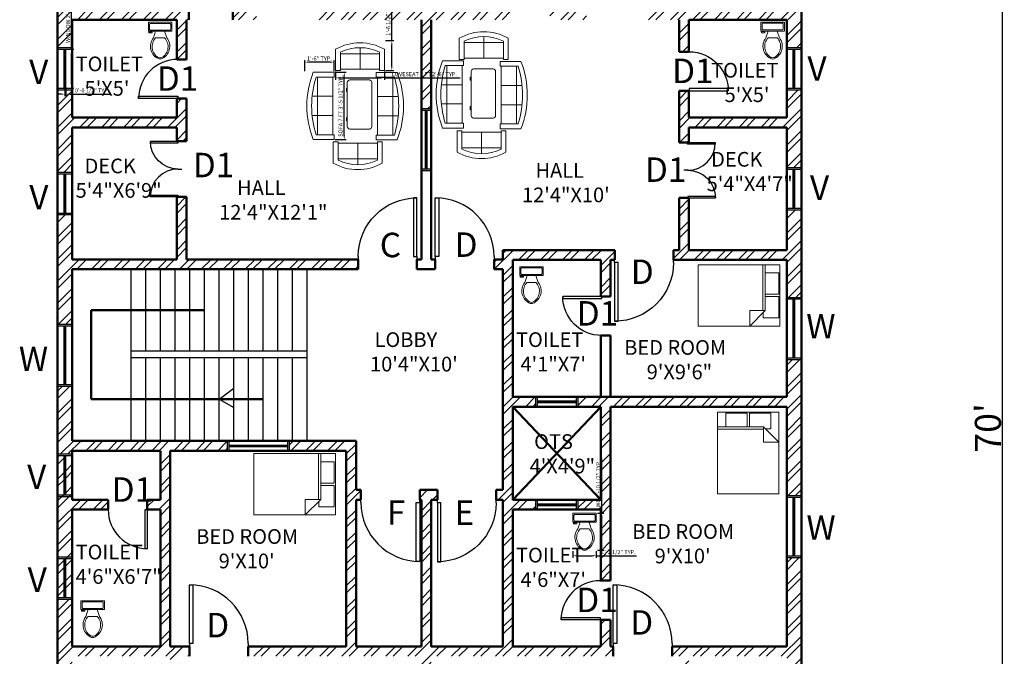
# Model space of a CAD drawing. Units: inches. Extents: x -31438 to -28352, y 12489 to 13610.
# Tile 2 of 5: x -31438 to -30834, y 12848 to 13238. Entities that reach past the tile are written whole.
import ezdxf

# ---------------------------------------------------------------- set-up
doc = ezdxf.new("R2010")
doc.units = ezdxf.units.IN
for name, color, linetype, lineweight in [('A-ANNO-DIMS', 2, 'Continuous', 18), ('A-ANNO-TEXT', 7, 'Continuous', 18), ('A-AREA-IDEN', 3, 'Continuous', 18), ('A-DOOR', 3, 'Continuous', 25), ('A-FLOR-FIXT', 9, 'Continuous', 18), ('A-FLOR-STRS', 6, 'Continuous', 25), ('A-FURN', 8, 'Continuous', 18), ('A-GLAZ', 4, 'Continuous', 25), ('A-WALL', 7, 'Continuous', 50), ('A-WALL-PATT', 8, 'Continuous', 13)]:
    doc.layers.add(name, color=color, linetype=linetype, lineweight=lineweight)
doc.styles.get("Standard").update_dxf_attribs({"font": 'arial.ttf'})
doc.dimstyles.new('ISO-25', dxfattribs={"dimtxt": 2.5, "dimasz": 2.5, "dimexe": 1.25, "dimexo": 0.625, "dimtad": 1, "dimdec": 0, "dimlunit": 3, "dimtxsty": 'Standard', "dimcen": 2.5, "dimadec": 0, "dimazin": 0, "dimtfac": 1, "dimtdec": 0, "dimtmove": 0, "dimatfit": 3, "dimfxl": 1, "dimarcsym": 0})

# ---------------------------------------------------------------- blocks, each defined once
blk = doc.blocks.new('*U8')
for p, q in [((0, 0), (0, -100)), ((750, 0), (750, -100))]:
    blk.add_line(p, q)
blk.add_lwpolyline([(0, 0), (0, 750), (43.75, 750), (43.75, 0)], close=True)
blk.add_arc((0, 0), 750, 0, 90)
blk = doc.blocks.new('Bed - Queen')
for p, q in [((0, -80.00003), (0, 0)), ((0, 0), (59.99999, 0)), ((59.99999, 0), (59.99999, -80.00003)), ((7.99999, -1.2), (28.79998, -1.2)), ((7.99999, -14.4), (7.99999, -1.2)), ((28.79998, -1.2), (28.79998, -14.4)), ((31.19999, -1.2), (51.99999, -1.2)), ((31.19999, -14.4), (31.19999, -1.2)), ((51.99999, -1.2), (51.99999, -16.4)), ((0, -14.4), (44.8, -14.4)), ((44.8, -16.8), (0, -16.8)), ((59.99999, -29.6), (44.8, -14.4)), ((44.8, -14.4), (44.8, -29.6)), ((51.99999, -16.4), (46.79936, -16.4)), ((44.8, -29.6), (59.99999, -29.6)), ((59.99999, -80.00003), (0, -80.00003))]:
    blk.add_line(p, q)
blk = doc.blocks.new('Desk - 30 x 60 in.')
for p, q in [((-26.999995, 0), (26.999995, 0)), ((-29.999995, -27), (-29.999995, -3)), ((29.999995, -3), (29.999995, -27)), ((26.999995, -30), (-26.999995, -30)), ((-20.000005, -30), (-20.000005, -31)), ((-20.000005, -31), (-16.000005, -31)), ((-16.000005, -31), (-16.000005, -30)), ((15.999995, -31), (15.999995, -30)), ((19.999995, -31), (15.999995, -31)), ((19.999995, -30), (19.999995, -31))]:
    blk.add_line(p, q)
for centre, start, end in [((-26.499995, -3.5), 98.1301, 171.8699), ((26.499995, -3.5), 8.130102, 81.8699), ((-26.499995, -26.5), 188.1301, 261.8699), ((26.499995, -26.5), 278.1301, 351.8699)]:
    blk.add_arc(centre, 3.535534, start, end)
blk = doc.blocks.new('Sofa - Roundback 7 ft.')
for p, q in [((-36.000027, -34), (-36.000027, -11.4696)), ((-12.00002, -32.4421), (-12.00003, -6.5971)), ((11.99997, -32.4421), (11.99998, -6.5971)), ((35.99998, -34), (35.99998, -11.4696)), ((-35.999844, -13.3819), (35.9998, -13.3819)), ((-36.000027, -32.4421), (35.99998, -32.4421))]:
    blk.add_line(p, q)
for points in [[(-36.000027, -34), (-42.000027, -34), (-42.000027, -8)], [(41.99998, -8), (41.99998, -34), (35.99998, -34)]]:
    blk.add_lwpolyline(points)
for centre, radius, start, end in [((0, -114.25), 114.25, 68.43141, 111.5686), ((-0.00001, -127.1968), 121.1968, 72.72033, 107.2797)]:
    blk.add_arc(centre, radius, start, end)
blk = doc.blocks.new('Sofa - Roundback Loveseat 5 ft.')
for p, q in [((-24, -33.99998), (-24, -11.46958)), ((0, -32.44198), (0, -5.99998)), ((24.00004, -33.99998), (24.00004, -11.46958)), ((-23.9998, -13.38178), (23.99986, -13.38178)), ((-24, -32.44198), (24.00004, -32.44198))]:
    blk.add_line(p, q)
for points in [[(-24, -33.99998), (-30, -33.99998), (-30, -7.99998)], [(30.00004, -7.99998), (30.00004, -33.99998), (24.00004, -33.99998)]]:
    blk.add_lwpolyline(points)
for centre, radius, start, end in [((0, -60.24998), 60.24998, 60.13715, 119.8628), ((0, -61.38438), 55.38444, 64.32083, 115.6792)]:
    blk.add_arc(centre, radius, start, end)
blk = doc.blocks.new('Toilet - top')
for p, q in [((-10, -8.5), (-8, -8.5)), ((-10, -9.5), (-10, -8.5)), ((-8, -8.5), (-8, -8)), ((-7, -8), (-7, -9.5)), ((-4, -8), (-6, -14)), ((4, -8), (6, -14)), ((9.5, -6), (9.5, -2)), ((-7, -9.5), (-10, -9.5)), ((4, -14), (-4, -14))]:
    blk.add_line(p, q)
blk.add_lwpolyline([(10.5, -8), (10.5, 0), (-10.5, 0), (-10.5, -8)], close=True)
for points in [[(-9.5, -2), (-9.5, -6)], [(8.5, -1), (-8.5, -1)], [(-8.5, -7), (8.5, -7)]]:
    blk.add_lwpolyline(points)
for centre, radius, start, end in [((-8.62, -1.88), 0.884, 81.8699, 188.1301), ((-8.62, -6.12), 0.884, 171.8699, 278.1301), ((8.62, -1.88), 0.884, 351.8699, 98.1301), ((8.62, -6.12), 0.884, 261.8699, 8.1301), ((3.52, -21.58), 12.17, 141.46911, 247.97143), ((4.2, -21.82), 11.33, 136.36773, 238.94682), ((-3.52, -21.58), 12.17, 292.02843, 38.53071), ((-4.2, -21.82), 11.33, 301.05301, 43.63209), ((0, -27.88), 4, 245.73182, 294.26817), ((0, -29), 4, 254.86053, 285.13947)]:
    blk.add_arc(centre, radius, start, end)
blk = doc.blocks.new('*D171')
at = {"layer": 'A-ANNO-DIMS', "color": 0, "lineweight": -2, "transparency": 16777216}
for p, q in [((-30958.23, 13407.92), (-30834.47, 13407.92)), ((-30835.72, 13405.42), (-30835.72, 12570.42)), ((-30958.23, 12567.92), (-30834.47, 12567.92))]:
    blk.add_line(p, q, dxfattribs=at)
at = {"layer": 'A-ANNO-DIMS', "color": 0, "transparency": 16777216}
for points in [[(-30836.13, 13405.42), (-30835.3, 13405.42), (-30835.72, 13407.92)], [(-30836.13, 12570.42), (-30835.3, 12570.42), (-30835.72, 12567.92)]]:
    blk.add_solid(points, dxfattribs=at)
at = {"layer": 'Defpoints', "color": 0, "transparency": 16777216}
for p in [(-30958.86, 13407.92), (-30958.86, 12567.92), (-30835.72, 12567.92)]:
    blk.add_point(p, dxfattribs=at)
at = {"layer": 'A-ANNO-DIMS', "color": 0, "transparency": 16777216, "insert": (-30844.51, 12987.92), "char_height": 2.5, "attachment_point": 5, "rotation": 90}
blk.add_mtext("{\\H6.4x;70'}", dxfattribs=at)
blk = doc.blocks.new('WIN-24')
for p, q in [((0, 0), (0, 24)), ((0.5, 0), (0.5, 24))]:
    blk.add_line(p, q)
blk = doc.blocks.new('WIN-36')
for p, q in [((0, 0), (0, 36)), ((0.5, 0), (0.5, 36))]:
    blk.add_line(p, q)
blk = doc.blocks.new('*D177')
at = {"layer": 'A-ANNO-DIMS', "color": 0, "lineweight": -2, "transparency": 16777216}
for p, q in [((-31244.72, 13205.88), (-31237.9, 13205.88)), ((-31239.15, 13167.1), (-31239.15, 13203.38)), ((-31244.72, 13164.6), (-31237.9, 13164.6))]:
    blk.add_line(p, q, dxfattribs=at)
at = {"layer": 'A-ANNO-DIMS', "color": 0, "transparency": 16777216}
for points in [[(-31239.57, 13203.38), (-31238.74, 13203.38), (-31239.15, 13205.88)], [(-31239.57, 13167.1), (-31238.74, 13167.1), (-31239.15, 13164.6)]]:
    blk.add_solid(points, dxfattribs=at)
at = {"layer": 'Defpoints', "color": 0, "transparency": 16777216}
for p in [(-31245.35, 13205.88), (-31239.15, 13205.88), (-31245.35, 13164.6)]:
    blk.add_point(p, dxfattribs=at)
at = {"layer": 'A-ANNO-DIMS', "color": 0, "transparency": 16777216, "insert": (-31241.07, 13185.24), "char_height": 2.5, "attachment_point": 5, "rotation": 90}
blk.add_mtext('SOFA 7 FT 3\'-5 1/2" TYP.', dxfattribs=at)
blk = doc.blocks.new('*D178')
at = {"layer": 'A-ANNO-DIMS', "color": 0, "lineweight": -2, "transparency": 16777216}
for p, q in [((-31263.37, 13206.51), (-31263.37, 13213.32)), ((-31247.85, 13212.07), (-31260.87, 13212.07)), ((-31245.35, 13206.51), (-31245.35, 13213.32))]:
    blk.add_line(p, q, dxfattribs=at)
at = {"layer": 'A-ANNO-DIMS', "color": 0, "transparency": 16777216}
for points in [[(-31260.87, 13212.49), (-31260.87, 13211.66), (-31263.37, 13212.07)], [(-31247.85, 13212.49), (-31247.85, 13211.66), (-31245.35, 13212.07)]]:
    blk.add_solid(points, dxfattribs=at)
at = {"layer": 'Defpoints', "color": 0, "transparency": 16777216}
for p in [(-31263.37, 13212.07), (-31263.37, 13205.88), (-31245.35, 13205.88)]:
    blk.add_point(p, dxfattribs=at)
at = {"layer": 'A-ANNO-DIMS', "color": 0, "transparency": 16777216, "insert": (-31254.36, 13213.98), "char_height": 2.5, "attachment_point": 5}
blk.add_mtext('1\'-6" TYP.', dxfattribs=at)
blk = doc.blocks.new('*D181')
at = {"layer": 'A-ANNO-DIMS', "color": 0, "lineweight": -2, "transparency": 16777216}
for p, q in [((-31244.46, 13206.33), (-31244.46, 13201.2)), ((-31241.96, 13202.45), (-31216.96, 13202.45)), ((-31214.46, 13206.33), (-31214.46, 13201.2)), ((-31214.46, 13202.45), (-31168.03, 13202.45))]:
    blk.add_line(p, q, dxfattribs=at)
at = {"layer": 'A-ANNO-DIMS', "color": 0, "transparency": 16777216}
for points in [[(-31241.96, 13202.87), (-31241.96, 13202.04), (-31244.46, 13202.45)], [(-31216.96, 13202.87), (-31216.96, 13202.04), (-31214.46, 13202.45)]]:
    blk.add_solid(points, dxfattribs=at)
at = {"layer": 'Defpoints', "color": 0, "transparency": 16777216}
for p in [(-31244.46, 13206.95), (-31214.46, 13206.95), (-31214.46, 13202.45)]:
    blk.add_point(p, dxfattribs=at)
at = {"layer": 'A-ANNO-DIMS', "color": 0, "transparency": 16777216, "insert": (-31189.99, 13204.37), "char_height": 2.5, "attachment_point": 5}
blk.add_mtext('LOVESEAT 5 FT 2\'-6" TYP.', dxfattribs=at)
blk = doc.blocks.new('*D182')
at = {"layer": 'A-ANNO-DIMS', "color": 0, "lineweight": -2, "transparency": 16777216}
for p, q in [((-31209.96, 13225.29), (-31209.96, 13249.87)), ((-31213.84, 13225.29), (-31208.71, 13225.29)), ((-31209.96, 13209.45), (-31209.96, 13222.79)), ((-31213.84, 13206.95), (-31208.71, 13206.95))]:
    blk.add_line(p, q, dxfattribs=at)
at = {"layer": 'A-ANNO-DIMS', "color": 0, "transparency": 16777216}
for points in [[(-31210.38, 13222.79), (-31209.55, 13222.79), (-31209.96, 13225.29)], [(-31210.38, 13209.45), (-31209.55, 13209.45), (-31209.96, 13206.95)]]:
    blk.add_solid(points, dxfattribs=at)
at = {"layer": 'Defpoints', "color": 0, "transparency": 16777216}
for p in [(-31214.46, 13225.29), (-31209.96, 13225.29), (-31214.46, 13206.95)]:
    blk.add_point(p, dxfattribs=at)
at = {"layer": 'A-ANNO-DIMS', "color": 0, "transparency": 16777216, "insert": (-31211.88, 13238.83), "char_height": 2.5, "attachment_point": 5, "rotation": 90}
blk.add_mtext('1\'-6 1/2" TYP.', dxfattribs=at)
blk = doc.blocks.new('*D189')
at = {"layer": 'A-ANNO-DIMS', "color": 0, "lineweight": -2, "transparency": 16777216}
for p, q in [((-31081.19, 12935.57), (-31081.19, 12969.22)), ((-31083.96, 12935.57), (-31079.94, 12935.57)), ((-31081.19, 12915.44), (-31081.19, 12933.07)), ((-31083.96, 12912.94), (-31079.94, 12912.94))]:
    blk.add_line(p, q, dxfattribs=at)
at = {"layer": 'A-ANNO-DIMS', "color": 0, "transparency": 16777216}
for points in [[(-31081.61, 12933.07), (-31080.78, 12933.07), (-31081.19, 12935.57)], [(-31081.61, 12915.44), (-31080.78, 12915.44), (-31081.19, 12912.94)]]:
    blk.add_solid(points, dxfattribs=at)
at = {"layer": 'Defpoints', "color": 0, "transparency": 16777216}
for p in [(-31084.59, 12935.57), (-31081.19, 12935.57), (-31084.59, 12912.94)]:
    blk.add_point(p, dxfattribs=at)
at = {"layer": 'A-ANNO-DIMS', "color": 0, "transparency": 16777216, "insert": (-31083.11, 12953.64), "char_height": 2.5, "attachment_point": 5, "rotation": 90}
blk.add_mtext('WC 1\'-10 1/2" TYP.', dxfattribs=at)
blk = doc.blocks.new('*D190')
at = {"layer": 'A-ANNO-DIMS', "color": 0, "lineweight": -2, "transparency": 16777216}
for p, q in [((-31098.97, 12912.31), (-31098.97, 12908.29)), ((-31084.59, 12912.31), (-31084.59, 12908.29)), ((-31096.47, 12909.54), (-31087.09, 12909.54)), ((-31084.59, 12909.54), (-31060.01, 12909.54))]:
    blk.add_line(p, q, dxfattribs=at)
at = {"layer": 'A-ANNO-DIMS', "color": 0, "transparency": 16777216}
for points in [[(-31096.47, 12909.96), (-31096.47, 12909.13), (-31098.97, 12909.54)], [(-31087.09, 12909.96), (-31087.09, 12909.13), (-31084.59, 12909.54)]]:
    blk.add_solid(points, dxfattribs=at)
at = {"layer": 'Defpoints', "color": 0, "transparency": 16777216}
for p in [(-31098.97, 12912.94), (-31084.59, 12912.94), (-31084.59, 12909.54)]:
    blk.add_point(p, dxfattribs=at)
at = {"layer": 'A-ANNO-DIMS', "color": 0, "transparency": 16777216, "insert": (-31071.05, 12911.46), "char_height": 2.5, "attachment_point": 5}
blk.add_mtext('1\'-2 1/2" TYP.', dxfattribs=at)
blk = doc.blocks.new('*D193')
at = {"layer": 'A-ANNO-DIMS', "color": 0, "lineweight": -2, "transparency": 16777216}
for p, q in [((-31406.26, 13220.1), (-31406.26, 13255.48)), ((-31409.23, 13220.1), (-31405.01, 13220.1)), ((-31406.26, 13198.6), (-31406.26, 13217.6)), ((-31409.23, 13196.1), (-31405.01, 13196.1))]:
    blk.add_line(p, q, dxfattribs=at)
at = {"layer": 'A-ANNO-DIMS', "color": 0, "transparency": 16777216}
for points in [[(-31406.67, 13217.6), (-31405.84, 13217.6), (-31406.26, 13220.1)], [(-31406.67, 13198.6), (-31405.84, 13198.6), (-31406.26, 13196.1)]]:
    blk.add_solid(points, dxfattribs=at)
at = {"layer": 'Defpoints', "color": 0, "transparency": 16777216}
for p in [(-31409.86, 13220.1), (-31406.26, 13220.1), (-31409.86, 13196.1)]:
    blk.add_point(p, dxfattribs=at)
at = {"layer": 'A-ANNO-DIMS', "color": 0, "transparency": 16777216, "insert": (-31408.17, 13239.04), "char_height": 2.5, "attachment_point": 5, "rotation": 90}
blk.add_mtext('WINDOW 2\'-0" TYP.', dxfattribs=at)
blk = doc.blocks.new('*D194')
at = {"layer": 'A-ANNO-DIMS', "color": 0, "lineweight": -2, "transparency": 16777216}
for p, q in [((-31412.86, 13192.5), (-31415.36, 13192.5)), ((-31410.36, 13195.47), (-31410.36, 13191.25)), ((-31410.36, 13192.5), (-31409.86, 13192.5)), ((-31409.86, 13195.47), (-31409.86, 13191.25)), ((-31407.36, 13192.5), (-31382.54, 13192.5))]:
    blk.add_line(p, q, dxfattribs=at)
at = {"layer": 'A-ANNO-DIMS', "color": 0, "transparency": 16777216}
for points in [[(-31412.86, 13192.91), (-31412.86, 13192.08), (-31410.36, 13192.5)], [(-31407.36, 13192.91), (-31407.36, 13192.08), (-31409.86, 13192.5)]]:
    blk.add_solid(points, dxfattribs=at)
at = {"layer": 'Defpoints', "color": 0, "transparency": 16777216}
for p in [(-31410.36, 13196.1), (-31409.86, 13196.1), (-31409.86, 13192.5)]:
    blk.add_point(p, dxfattribs=at)
at = {"layer": 'A-ANNO-DIMS', "color": 0, "transparency": 16777216, "insert": (-31393.7, 13194.41), "char_height": 2.5, "attachment_point": 5}
blk.add_mtext('0\'-0 1/2" TYP.', dxfattribs=at)

msp = doc.modelspace()

# ---------------------------------------------------------------- hatches: boundary and pattern name
at = {"layer": 'A-WALL-PATT'}
h = msp.add_hatch(dxfattribs=at)
h.set_pattern_fill('ANSI32', color=256)
h.paths.add_polyline_path([(-30958.86, 13431.92), (-30992.36, 13431.92), (-30992.36, 13425.92), (-30964.86, 13425.92), (-30964.86, 13383.92), (-31006.63, 13383.92), (-31006.63, 13380.92), (-31006.63, 13377.92), (-30958.86, 13377.92)])
h.paths.add_polyline_path([(-30958.86, 13377.92), (-30967.86, 13377.92), (-30967.86, 13330.01), (-30958.86, 13330.01)])
h.paths.add_polyline_path([(-31018.36, 13431.92), (-31051.86, 13431.92), (-31051.86, 13407.92), (-31124.86, 13407.92), (-31124.86, 13398.92), (-31101.86, 13398.92), (-31101.86, 13362.92), (-31185.86, 13362.92), (-31185.86, 13398.92), (-31162.86, 13398.92), (-31162.86, 13407.92), (-31185.86, 13407.92), (-31185.86, 13431.92), (-31217.86, 13431.92), (-31217.86, 13425.92), (-31191.86, 13425.92), (-31191.86, 13383.92), (-31230.51, 13383.92), (-31230.51, 13377.92), (-31191.86, 13377.92), (-31191.86, 13244.1), (-31256.99, 13244.1), (-31256.99, 13238.1), (-31191.86, 13238.1), (-31191.86, 13183.6), (-31185.86, 13183.6), (-31185.86, 13238.1), (-31137.12, 13238.1), (-31137.12, 13244.1), (-31185.86, 13244.1), (-31185.86, 13356.92), (-31101.86, 13356.92), (-31101.86, 13340.51), (-31095.86, 13340.51), (-31095.86, 13398.92), (-31051.86, 13398.92), (-31051.86, 13377.92), (-31030.63, 13377.92), (-31030.63, 13383.92), (-31045.86, 13383.92), (-31045.86, 13425.92), (-31018.36, 13425.92)])
h.paths.add_polyline_path([(-31269.86, 13425.92), (-31243.86, 13425.92), (-31243.86, 13431.92), (-31275.86, 13431.92), (-31275.86, 13407.92), (-31336.86, 13407.92), (-31336.86, 13398.92), (-31305.86, 13398.92), (-31305.86, 13362.92), (-31405.86, 13362.92), (-31405.86, 13398.92), (-31374.86, 13398.92), (-31374.86, 13407.92), (-31414.86, 13407.92), (-31414.86, 13340.51), (-31405.86, 13340.51), (-31405.86, 13356.92), (-31305.86, 13356.92), (-31305.86, 13340.51), (-31299.86, 13340.51), (-31299.86, 13398.92), (-31275.86, 13398.92), (-31275.86, 13377.92), (-31254.51, 13377.92), (-31254.51, 13383.92), (-31269.86, 13383.92)])
h.paths.add_polyline_path([(-31299.86, 13302.51), (-31305.86, 13302.51), (-31305.86, 13244.1), (-31307.44, 13244.1), (-31307.44, 13241.1), (-31307.44, 13238.1), (-31292.99, 13238.1), (-31292.99, 13244.1), (-31299.86, 13244.1)])
h.paths.add_polyline_path([(-31334.44, 13244.1), (-31405.86, 13244.1), (-31405.86, 13302.51), (-31414.86, 13302.51), (-31414.86, 13221.1), (-31405.86, 13221.1), (-31405.86, 13238.1), (-31341.86, 13238.1), (-31341.86, 13213.77), (-31335.86, 13213.77), (-31335.86, 13238.1), (-31334.44, 13238.1)])
h.paths.add_polyline_path([(-31090.53, 13244.1), (-31095.86, 13244.1), (-31095.86, 13302.51), (-31101.86, 13302.51), (-31101.86, 13244.1), (-31113.12, 13244.1), (-31113.12, 13241.1), (-31113.12, 13238.1), (-31090.53, 13238.1)], flags=17)
h.paths.add_polyline_path([(-30958.86, 13292.01), (-30967.86, 13292.01), (-30967.86, 13244.1), (-31033.86, 13244.1), (-31054.53, 13244.1), (-31054.53, 13241.1), (-31054.53, 13238.1), (-31033.86, 13238.1), (-31033.86, 13218.45), (-31027.86, 13218.45), (-31027.86, 13238.1), (-30967.86, 13238.1), (-30967.86, 13221.1), (-30958.86, 13221.1)])
h.paths.add_polyline_path([(-30958.86, 13195.1), (-30967.86, 13195.1), (-30967.86, 13178.1), (-31027.86, 13178.1), (-31027.86, 13194.45), (-31030.86, 13194.45), (-31033.86, 13194.45), (-31033.86, 13162.82), (-31027.86, 13162.82), (-31027.86, 13172.1), (-30967.86, 13172.1), (-30967.86, 13147.51), (-30958.86, 13147.51)])
h.paths.add_polyline_path([(-30958.86, 13121.51), (-30967.86, 13121.51), (-30967.86, 13096.92), (-31027.86, 13096.92), (-31027.86, 13128.82), (-31033.86, 13128.82), (-31033.86, 13096.92), (-31037.31, 13096.92), (-31037.31, 13090.92), (-30967.86, 13090.92), (-30967.86, 13067.92), (-30958.86, 13067.92)])
h.paths.add_polyline_path([(-30958.86, 13029.92), (-30967.86, 13029.92), (-30967.86, 13006.92), (-31025.37, 13006.92), (-31095.86, 13006.92), (-31095.86, 13000.92), (-31081.86, 13000.92), (-31081.86, 12943.92), (-31095.86, 12943.92), (-31095.86, 12937.92), (-31081.86, 12937.92), (-31081.86, 12894.3), (-31075.86, 12894.3), (-31075.86, 13000.92), (-31025.37, 13000.92), (-30967.86, 13000.92), (-30967.86, 12946.42), (-30958.86, 12946.42)])
h.paths.add_polyline_path([(-31121.86, 13006.92), (-31135.86, 13006.92), (-31135.86, 13090.92), (-31081.86, 13090.92), (-31081.86, 13068.53), (-31075.86, 13068.53), (-31075.86, 13090.92), (-31073.31, 13090.92), (-31073.31, 13096.92), (-31141.86, 13096.92), (-31141.86, 13091.1), (-31147.29, 13091.1), (-31147.29, 13085.1), (-31141.86, 13085.1), (-31141.86, 12949.88), (-31146.05, 12949.88), (-31146.05, 12943.88), (-31141.86, 12943.88), (-31141.86, 12853.92), (-31185.86, 12853.92), (-31185.86, 12943.88), (-31182.05, 12943.88), (-31182.05, 12949.88), (-31192.89, 12949.88), (-31192.89, 12943.88), (-31191.86, 12943.88), (-31191.86, 12853.92), (-31231.86, 12853.92), (-31231.86, 12943.88), (-31228.89, 12943.88), (-31228.89, 12949.88), (-31231.86, 12949.88), (-31231.86, 12979.92), (-31272.86, 12979.92), (-31272.86, 12973.92), (-31237.86, 12973.92), (-31237.86, 12853.92), (-31298, 12853.92), (-31298, 12847.92), (-31191.86, 12847.92), (-31191.86, 12806.42), (-31185.86, 12806.42), (-31185.86, 12847.92), (-31074.17, 12847.92), (-31074.17, 12853.92), (-31075.86, 12853.92), (-31075.86, 12870.3), (-31081.86, 12870.3), (-31081.86, 12853.92), (-31135.86, 12853.92), (-31135.86, 12937.92), (-31121.86, 12937.92), (-31121.86, 12943.92), (-31135.86, 12943.92), (-31135.86, 13000.92), (-31121.86, 13000.92)])
h.paths.add_polyline_path([(-30958.86, 12908.42), (-30967.86, 12908.42), (-30967.86, 12853.92), (-31038.17, 12853.92), (-31038.17, 12850.92), (-31038.17, 12847.92), (-31033.86, 12847.92), (-31033.86, 12837.06), (-31027.86, 12837.06), (-31027.86, 12847.92), (-30967.86, 12847.92), (-30967.86, 12833.42), (-30958.86, 12833.42)])
h.paths.add_polyline_path([(-30958.86, 12807.42), (-30967.86, 12807.42), (-30967.86, 12792.92), (-31027.86, 12792.92), (-31027.86, 12803.06), (-31033.86, 12803.06), (-31033.86, 12773.49), (-31027.86, 12773.49), (-31027.86, 12786.92), (-30967.86, 12786.92), (-30967.86, 12769.92), (-30958.86, 12769.92)])
h.paths.add_polyline_path([(-30958.86, 12743.92), (-30967.86, 12743.92), (-30967.86, 12726.92), (-31027.86, 12726.92), (-31027.86, 12749.49), (-31033.86, 12749.49), (-31033.86, 12726.92), (-31035.47, 12726.92), (-31035.47, 12720.92), (-30967.86, 12720.92), (-30967.86, 12667.92), (-30958.86, 12667.92)])
h.paths.add_polyline_path([(-30958.86, 12629.92), (-30967.86, 12629.92), (-30967.86, 12618.92), (-31071.86, 12618.92), (-31071.86, 12612.92), (-30967.86, 12612.92), (-30967.86, 12576.92), (-31000.86, 12576.92), (-31000.86, 12567.92), (-30958.86, 12567.92)])
h.paths.add_polyline_path([(-31038.86, 12576.92), (-31071.86, 12576.92), (-31071.86, 12629.92), (-31077.86, 12629.92), (-31077.86, 12576.92), (-31101.86, 12576.92), (-31101.86, 12597.92), (-31115.03, 12597.92), (-31115.03, 12591.92), (-31107.86, 12591.92), (-31107.86, 12549.92), (-31133.86, 12549.92), (-31133.86, 12543.92), (-31101.86, 12543.92), (-31101.86, 12567.92), (-31038.86, 12567.92)])
h.paths.add_polyline_path([(-31159.86, 12549.92), (-31185.86, 12549.92), (-31185.86, 12591.92), (-31139.03, 12591.92), (-31139.03, 12597.92), (-31185.86, 12597.92), (-31185.86, 12720.92), (-31126.49, 12720.92), (-31126.49, 12726.92), (-31185.86, 12726.92), (-31185.86, 12768.42), (-31191.86, 12768.42), (-31191.86, 12726.92), (-31226.35, 12726.92), (-31226.35, 12720.92), (-31191.86, 12720.92), (-31191.86, 12618.92), (-31275.86, 12618.92), (-31275.86, 12720.92), (-31262.35, 12720.92), (-31262.35, 12726.92), (-31298.57, 12726.92), (-31298.57, 12720.92), (-31281.86, 12720.92), (-31281.86, 12576.92), (-31321.86, 12576.92), (-31321.86, 12597.92), (-31340.38, 12597.92), (-31340.38, 12591.92), (-31327.86, 12591.92), (-31327.86, 12549.92), (-31355.36, 12549.92), (-31355.36, 12543.92), (-31321.86, 12543.92), (-31321.86, 12567.92), (-31252.86, 12567.92), (-31252.86, 12576.92), (-31275.86, 12576.92), (-31275.86, 12612.92), (-31191.86, 12612.92), (-31191.86, 12576.92), (-31214.86, 12576.92), (-31214.86, 12567.92), (-31191.86, 12567.92), (-31191.86, 12543.92), (-31159.86, 12543.92)])
h.paths.add_polyline_path([(-31071.86, 12720.92), (-31071.47, 12726.92), (-31090.49, 12726.92), (-31090.49, 12720.92), (-31077.86, 12720.92), (-31077.86, 12667.92), (-31071.86, 12667.92)])
h.paths.add_polyline_path([(-31381.36, 12549.92), (-31408.86, 12549.92), (-31408.86, 12591.92), (-31364.38, 12591.92), (-31364.38, 12597.92), (-31414.86, 12597.92), (-31414.86, 12543.92), (-31381.36, 12543.92)])
h.paths.add_polyline_path([(-31405.86, 12640.42), (-31414.86, 12640.42), (-31414.86, 12597.92), (-31405.86, 12597.92)])
h.paths.add_polyline_path([(-31405.86, 12720.92), (-31334.57, 12720.92), (-31334.57, 12726.92), (-31339.86, 12726.92), (-31339.86, 12750.16), (-31345.86, 12750.16), (-31345.86, 12726.92), (-31405.86, 12726.92), (-31405.86, 12743.92), (-31414.86, 12743.92), (-31414.86, 12678.42), (-31405.86, 12678.42)])
h.paths.add_polyline_path([(-31339.86, 12806.09), (-31345.86, 12806.09), (-31345.86, 12792.92), (-31405.86, 12792.92), (-31405.86, 12807.42), (-31414.86, 12807.42), (-31414.86, 12769.92), (-31405.86, 12769.92), (-31405.86, 12786.92), (-31345.86, 12786.92), (-31345.86, 12774.16), (-31339.86, 12774.16)])
h.paths.add_polyline_path([(-31334, 12853.92), (-31345.86, 12853.92), (-31345.86, 12973.92), (-31310.86, 12973.92), (-31310.86, 12979.92), (-31405.86, 12979.92), (-31405.86, 13013.51), (-31414.86, 13013.51), (-31414.86, 12971.92), (-31405.86, 12971.92), (-31405.86, 12970.92), (-31409.86, 12970.92), (-31409.86, 12946.92), (-31410.86, 12946.92), (-31410.86, 12970.92), (-31414.86, 12970.92), (-31414.86, 12883.92), (-31405.86, 12883.92), (-31405.86, 12882.92), (-31414.86, 12882.92), (-31414.86, 12833.42), (-31405.86, 12833.42), (-31405.86, 12847.92), (-31345.86, 12847.92), (-31345.86, 12840.09), (-31339.86, 12840.09), (-31339.86, 12847.92), (-31334, 12847.92)])
h.paths.add_polyline_path([(-31351.86, 12937.92), (-31359.89, 12937.92), (-31359.89, 12943.92), (-31351.86, 12943.92), (-31351.86, 12973.92), (-31405.86, 12973.92), (-31405.86, 12943.92), (-31383.89, 12943.92), (-31383.89, 12937.92), (-31405.86, 12937.92), (-31405.86, 12853.92), (-31351.86, 12853.92)], flags=16)
h.paths.add_polyline_path([(-31386.16, 12876.52), (-31390.61, 12876.52), (-31389.24, 12872.41, -0.501323), (-31392.64, 12859.49, -0.132891), (-31394.07, 12859.49, -0.501317), (-31397.46, 12872.41), (-31396.09, 12876.52), (-31398.15, 12876.52), (-31398.15, 12875.49), (-31400.2, 12875.49), (-31400.2, 12876.18), (-31400.22, 12876.52), (-31400.54, 12876.52), (-31400.54, 12882), (-31386.16, 12882)], flags=0)
h.paths.add_polyline_path([(-31387.36, 12877.2), (-31399.17, 12877.2, -0.414214), (-31399.86, 12877.72), (-31399.86, 12880.63, -0.414214), (-31399.35, 12881.31), (-31387.53, 12881.31, -0.414214), (-31386.85, 12880.8), (-31386.85, 12877.89, -0.414214)], flags=0)
h.paths.add_polyline_path([(-31392.23, 12860.41, -0.215004), (-31394.48, 12860.41, -0.48008), (-31396.09, 12872.41), (-31390.61, 12872.41, -0.48008)], flags=0)
h.paths.add_polyline_path([(-31359.87, 12913.86), (-31361.27, 12913.86), (-31361.27, 12937.86), (-31359.87, 12937.86)], flags=0)
h.paths.add_polyline_path([(-31230.55, 13091.1), (-31335.86, 13091.1), (-31335.86, 13129.57), (-31341.86, 13129.57), (-31341.86, 13091.1), (-31405.86, 13091.1), (-31405.86, 13118.6), (-31414.86, 13118.6), (-31414.86, 13051.51), (-31405.86, 13051.51), (-31405.86, 13085.1), (-31230.55, 13085.1)])
h.paths.add_polyline_path([(-31335.86, 13189.77), (-31341.86, 13189.77), (-31341.86, 13178.1), (-31405.86, 13178.1), (-31405.86, 13195.1), (-31414.86, 13195.1), (-31414.86, 13144.6), (-31405.86, 13144.6), (-31405.86, 13172.1), (-31341.86, 13172.1), (-31341.86, 13163.57), (-31335.86, 13163.57)])
h.paths.add_polyline_path([(-31387.11, 12934.37), (-31352.82, 12934.37), (-31352.82, 12965.28), (-31387.11, 12965.28)], flags=8)
h.paths.add_polyline_path([(-31406.38, 12887.22), (-31351.66, 12887.22), (-31351.66, 12920.8), (-31406.38, 12920.8)], flags=24)

# ---------------------------------------------------------------- linework, layer by layer
at = {"layer": 'A-FLOR-STRS'}
for p, q in [((-31369.86, 12979.92), (-31369.86, 13085.1)), ((-31360.86, 13034.92), (-31360.86, 13085.1)), ((-31351.86, 13034.92), (-31351.86, 13085.1)), ((-31342.86, 13034.92), (-31342.86, 13085.1)), ((-31333.86, 13034.92), (-31333.86, 13085.1)), ((-31324.86, 13034.92), (-31324.86, 13085.1)), ((-31315.86, 13034.92), (-31315.86, 13085.1)), ((-31306.86, 13034.92), (-31306.86, 13085.1)), ((-31297.86, 13034.92), (-31297.86, 13085.1)), ((-31288.86, 13034.92), (-31288.86, 13085.1)), ((-31279.86, 13034.92), (-31279.86, 13085.1)), ((-31270.86, 13034.92), (-31270.86, 13085.1)), ((-31261.86, 12979.92), (-31261.86, 13085.1)), ((-31261.86, 13034.92), (-31369.86, 13034.92)), ((-31261.86, 13030.92), (-31369.86, 13030.92)), ((-31360.86, 12979.92), (-31360.86, 13030.92)), ((-31351.86, 12979.92), (-31351.86, 13030.92)), ((-31342.86, 12979.92), (-31342.86, 13030.92)), ((-31333.86, 12979.92), (-31333.86, 13030.92)), ((-31324.86, 12979.92), (-31324.86, 13030.92)), ((-31315.86, 12979.92), (-31315.86, 13030.92)), ((-31306.86, 12979.92), (-31306.86, 13030.92)), ((-31297.86, 12979.92), (-31297.86, 13030.92)), ((-31288.86, 12979.92), (-31288.86, 13030.92)), ((-31279.86, 12979.92), (-31279.86, 13030.92)), ((-31270.86, 12979.92), (-31270.86, 13030.92)), ((-31315.86, 13005.42), (-31306.86, 13012.36)), ((-31315.86, 13005.42), (-31306.86, 13000.42)), ((-31309.86, 12977.42), (-31273.86, 12977.42)), ((-31309.86, 12976.92), (-31273.86, 12976.92)), ((-31309.86, 12976.42), (-31273.86, 12976.42))]:
    msp.add_line(p, q, dxfattribs=at)
at = {"layer": 'A-GLAZ'}
for p, q in [((-31414.86, 13221.1), (-31405.86, 13221.1)), ((-31414.86, 13220.1), (-31405.86, 13220.1)), ((-31410.86, 13196.1), (-31410.86, 13220.1)), ((-30967.86, 13221.1), (-30958.86, 13221.1)), ((-30967.86, 13220.1), (-30958.86, 13220.1)), ((-30963.86, 13196.1), (-30963.86, 13220.1)), ((-31414.86, 13196.1), (-31405.86, 13196.1)), ((-30967.86, 13196.1), (-30958.86, 13196.1)), ((-31414.86, 13195.1), (-31405.86, 13195.1)), ((-30967.86, 13195.1), (-30958.86, 13195.1)), ((-31191.86, 13183.6), (-31185.86, 13183.6)), ((-31191.86, 13182.6), (-31185.86, 13182.6)), ((-31189.36, 13146.6), (-31189.36, 13182.6)), ((-31188.86, 13146.6), (-31188.86, 13182.6)), ((-31188.36, 13146.6), (-31188.36, 13182.6)), ((-30967.86, 13147.51), (-30958.86, 13147.51)), ((-31414.86, 13144.6), (-31405.86, 13144.6)), ((-31414.86, 13143.6), (-31405.86, 13143.6)), ((-31410.86, 13119.6), (-31410.86, 13143.6)), ((-31191.86, 13146.6), (-31185.86, 13146.6)), ((-31191.86, 13145.6), (-31185.86, 13145.6)), ((-30967.86, 13146.51), (-30958.86, 13146.51)), ((-30963.86, 13122.51), (-30963.86, 13146.51)), ((-31414.86, 13119.6), (-31405.86, 13119.6)), ((-31414.86, 13118.6), (-31405.86, 13118.6)), ((-30967.86, 13122.51), (-30958.86, 13122.51)), ((-30967.86, 13121.51), (-30958.86, 13121.51)), ((-30967.86, 13067.92), (-30958.86, 13067.92)), ((-30967.86, 13066.92), (-30958.86, 13066.92)), ((-30963.86, 13030.92), (-30963.86, 13066.92)), ((-31414.86, 13051.51), (-31405.86, 13051.51)), ((-31414.86, 13050.51), (-31405.86, 13050.51)), ((-31410.86, 13014.51), (-31410.86, 13050.51)), ((-30967.86, 13030.92), (-30958.86, 13030.92)), ((-30967.86, 13029.92), (-30958.86, 13029.92)), ((-31414.86, 13014.51), (-31405.86, 13014.51)), ((-31414.86, 13013.51), (-31405.86, 13013.51)), ((-31121.86, 13006.92), (-31121.86, 13000.92)), ((-31120.86, 13006.92), (-31120.86, 13000.92)), ((-31120.86, 13004.42), (-31096.86, 13004.42)), ((-31120.86, 13003.92), (-31096.86, 13003.92)), ((-31120.86, 13003.42), (-31096.86, 13003.42)), ((-31096.86, 13006.92), (-31096.86, 13000.92)), ((-31095.86, 13006.92), (-31095.86, 13000.92)), ((-31310.86, 12979.92), (-31310.86, 12973.92)), ((-31309.86, 12979.92), (-31309.86, 12973.92)), ((-31273.86, 12979.92), (-31273.86, 12973.92)), ((-31272.86, 12979.92), (-31272.86, 12973.92)), ((-31414.86, 12971.92), (-31405.86, 12971.92)), ((-31414.86, 12970.92), (-31405.86, 12970.92)), ((-31410.86, 12946.92), (-31410.86, 12970.92)), ((-31414.86, 12946.92), (-31405.86, 12946.92)), ((-31414.86, 12945.92), (-31405.86, 12945.92)), ((-31121.86, 12943.92), (-31121.86, 12937.92)), ((-31120.86, 12943.92), (-31120.86, 12937.92)), ((-31096.86, 12943.92), (-31096.86, 12937.92)), ((-31095.86, 12943.92), (-31095.86, 12937.92)), ((-30967.86, 12946.42), (-30958.86, 12946.42)), ((-30967.86, 12945.42), (-30958.86, 12945.42)), ((-30963.86, 12909.42), (-30963.86, 12945.42)), ((-31120.86, 12941.42), (-31096.86, 12941.42)), ((-31414.86, 12908.92), (-31405.86, 12908.92)), ((-31414.86, 12907.92), (-31405.86, 12907.92)), ((-31410.86, 12883.92), (-31410.86, 12907.92)), ((-30967.86, 12909.42), (-30958.86, 12909.42)), ((-30967.86, 12908.42), (-30958.86, 12908.42)), ((-31414.86, 12883.92), (-31405.86, 12883.92)), ((-31414.86, 12882.92), (-31405.86, 12882.92))]:
    msp.add_line(p, q, dxfattribs=at)
at = {"layer": 'A-WALL'}
for p, q in [((-30958.86, 13431.92), (-30958.86, 12567.92)), ((-31414.86, 12543.92), (-31414.86, 13407.92)), ((-31334.44, 13244.1), (-31334.44, 13238.1)), ((-31307.44, 13244.1), (-31307.44, 13238.1)), ((-31405.86, 13178.1), (-31405.86, 13238.1)), ((-31341.86, 13238.1), (-31405.86, 13238.1)), ((-31341.86, 13213.77), (-31341.86, 13238.1)), ((-31335.86, 13213.77), (-31335.86, 13238.1)), ((-31191.86, 13091.1), (-31191.86, 13238.1)), ((-31185.86, 13091.1), (-31185.86, 13238.1)), ((-31033.86, 13238.1), (-31033.86, 13218.45)), ((-30967.86, 13238.1), (-31027.86, 13238.1)), ((-31027.86, 13238.1), (-31027.86, 13218.45)), ((-30967.86, 13238.1), (-30967.86, 13178.1)), ((-31341.86, 13213.77), (-31335.86, 13213.77)), ((-31033.86, 13218.45), (-31027.86, 13218.45)), ((-31341.86, 13178.1), (-31341.86, 13189.77)), ((-31341.86, 13189.77), (-31335.86, 13189.77)), ((-31335.86, 13163.57), (-31335.86, 13189.77)), ((-31033.86, 13194.45), (-31027.86, 13194.45)), ((-31033.86, 13194.45), (-31033.86, 13162.82)), ((-31027.86, 13194.45), (-31027.86, 13178.1)), ((-31341.86, 13178.1), (-31405.86, 13178.1)), ((-31341.86, 13178.1), (-31405.86, 13178.1)), ((-30967.86, 13178.1), (-31027.86, 13178.1)), ((-31341.86, 13172.1), (-31405.86, 13172.1)), ((-31341.86, 13172.1), (-31405.86, 13172.1)), ((-31405.86, 13091.1), (-31405.86, 13172.1)), ((-31341.86, 13163.57), (-31341.86, 13172.1)), ((-30967.86, 13172.1), (-31027.86, 13172.1)), ((-31027.86, 13172.1), (-31027.86, 13162.82)), ((-30967.86, 13172.1), (-30967.86, 13096.92)), ((-31341.86, 13163.57), (-31335.86, 13163.57)), ((-31033.86, 13162.82), (-31027.86, 13162.82)), ((-31341.86, 13091.1), (-31341.86, 13129.57)), ((-31341.86, 13129.57), (-31335.86, 13129.57)), ((-31335.86, 13091.1), (-31335.86, 13129.57)), ((-31033.86, 13128.82), (-31027.86, 13128.82)), ((-31033.86, 13128.82), (-31033.86, 13096.92)), ((-31027.86, 13128.82), (-31027.86, 13096.92)), ((-31141.86, 13096.92), (-31141.86, 13091.1)), ((-31073.31, 13096.92), (-31141.86, 13096.92)), ((-31073.31, 13096.92), (-31073.31, 13090.92)), ((-31033.86, 13096.92), (-31037.31, 13096.92)), ((-31037.31, 13096.92), (-31037.31, 13090.92)), ((-30967.86, 13096.92), (-31027.86, 13096.92)), ((-31341.86, 13091.1), (-31405.86, 13091.1)), ((-31230.55, 13091.1), (-31335.86, 13091.1)), ((-31230.55, 13091.1), (-31230.55, 13085.1)), ((-31191.86, 13091.1), (-31194.55, 13091.1)), ((-31194.55, 13091.1), (-31194.55, 13085.1)), ((-31183.29, 13091.1), (-31185.86, 13091.1)), ((-31183.29, 13091.1), (-31183.29, 13085.1)), ((-31141.86, 13091.1), (-31147.29, 13091.1)), ((-31147.29, 13091.1), (-31147.29, 13085.1)), ((-31135.86, 13090.92), (-31135.86, 13006.92)), ((-31081.86, 13090.92), (-31135.86, 13090.92)), ((-31081.86, 13090.92), (-31081.86, 13068.53)), ((-31075.86, 13090.92), (-31075.86, 13068.53)), ((-31073.31, 13090.92), (-31075.86, 13090.92)), ((-30967.86, 13090.92), (-31037.31, 13090.92)), ((-30967.86, 13090.92), (-30967.86, 13006.92)), ((-31405.86, 12979.92), (-31405.86, 13085.1)), ((-31230.55, 13085.1), (-31405.86, 13085.1)), ((-31183.29, 13085.1), (-31194.55, 13085.1)), ((-31141.86, 13085.1), (-31147.29, 13085.1)), ((-31141.86, 13085.1), (-31141.86, 12949.88)), ((-31081.86, 13068.53), (-31075.86, 13068.53)), ((-31324.86, 13060.01), (-31394.25, 13060.01)), ((-31394.25, 13060.01), (-31394.25, 13005.42)), ((-31081.86, 13044.53), (-31075.86, 13044.53)), ((-31081.86, 13044.53), (-31081.86, 13006.92)), ((-31075.86, 13044.53), (-31075.86, 13006.92)), ((-31394.25, 13005.42), (-31288.86, 13005.42)), ((-31025.37, 13006.92), (-31135.86, 13006.92)), ((-30967.86, 13006.92), (-31025.37, 13006.92)), ((-31081.86, 13000.92), (-31135.86, 13000.92)), ((-31135.86, 13000.92), (-31135.86, 12943.92)), ((-31081.86, 13000.92), (-31135.86, 12943.92)), ((-31135.86, 13000.92), (-31081.86, 12943.92)), ((-31081.86, 13000.92), (-31081.86, 12943.92)), ((-31075.86, 13000.92), (-31075.86, 12894.3)), ((-31025.37, 13000.92), (-31075.86, 13000.92)), ((-30967.86, 13000.92), (-31025.37, 13000.92)), ((-30967.86, 13000.92), (-30967.86, 12853.92)), ((-31231.86, 12979.92), (-31405.86, 12979.92)), ((-31231.86, 12949.88), (-31231.86, 12979.92)), ((-31405.86, 12943.92), (-31405.86, 12973.92)), ((-31351.86, 12973.92), (-31405.86, 12973.92)), ((-31351.86, 12943.92), (-31351.86, 12973.92)), ((-31237.86, 12973.92), (-31345.86, 12973.92)), ((-31345.86, 12853.92), (-31345.86, 12973.92)), ((-31237.86, 12853.92), (-31237.86, 12973.92)), ((-31228.89, 12949.88), (-31231.86, 12949.88)), ((-31228.89, 12949.88), (-31228.89, 12943.88)), ((-31192.89, 12949.88), (-31192.89, 12943.88)), ((-31182.05, 12949.88), (-31192.89, 12949.88)), ((-31182.05, 12949.88), (-31182.05, 12943.88)), ((-31141.86, 12949.88), (-31146.05, 12949.88)), ((-31146.05, 12949.88), (-31146.05, 12943.88)), ((-31383.89, 12943.92), (-31405.86, 12943.92)), ((-31383.89, 12943.92), (-31383.89, 12937.92)), ((-31351.86, 12943.92), (-31359.89, 12943.92)), ((-31359.89, 12943.92), (-31359.89, 12937.92)), ((-31231.86, 12853.92), (-31231.86, 12943.88)), ((-31228.89, 12943.88), (-31231.86, 12943.88)), ((-31191.86, 12943.88), (-31192.89, 12943.88)), ((-31191.86, 12853.92), (-31191.86, 12943.88)), ((-31185.86, 12853.92), (-31185.86, 12943.88)), ((-31182.05, 12943.88), (-31185.86, 12943.88)), ((-31141.86, 12943.88), (-31146.05, 12943.88)), ((-31141.86, 12943.88), (-31141.86, 12853.92)), ((-31081.86, 12943.92), (-31135.86, 12943.92)), ((-31405.86, 12853.92), (-31405.86, 12937.92)), ((-31383.89, 12937.92), (-31405.86, 12937.92)), ((-31351.86, 12937.92), (-31359.89, 12937.92)), ((-31351.86, 12853.92), (-31351.86, 12937.92)), ((-31081.86, 12937.92), (-31135.86, 12937.92)), ((-31135.86, 12937.92), (-31135.86, 12853.92)), ((-31081.86, 12937.92), (-31081.86, 12894.3)), ((-31081.86, 12894.3), (-31075.86, 12894.3)), ((-31081.86, 12870.3), (-31075.86, 12870.3)), ((-31081.86, 12870.3), (-31081.86, 12853.92)), ((-31075.86, 12870.3), (-31075.86, 12853.92)), ((-31351.86, 12853.92), (-31405.86, 12853.92)), ((-31334, 12853.92), (-31345.86, 12853.92)), ((-31334, 12853.92), (-31334, 12847.92)), ((-31237.86, 12853.92), (-31298, 12853.92)), ((-31298, 12853.92), (-31298, 12847.92)), ((-31191.86, 12853.92), (-31231.86, 12853.92)), ((-31141.86, 12853.92), (-31185.86, 12853.92)), ((-31081.86, 12853.92), (-31135.86, 12853.92)), ((-31074.17, 12853.92), (-31075.86, 12853.92)), ((-31074.17, 12853.92), (-31074.17, 12847.92)), ((-30967.86, 12853.92), (-31038.17, 12853.92)), ((-31038.17, 12853.92), (-31038.17, 12847.92))]:
    msp.add_line(p, q, dxfattribs=at)

# ---------------------------------------------------------------- block references
at = {"layer": 'A-DOOR'}
for p, xscale, yscale, zscale, rotation in [((-31341.22, 13189.8), 0.0319618796001435, 0.0319618796001435, 0.0319618796001435, 90), ((-31027.66, 13194.45), -0.0320000000000053, 0.0320000000000053, 0.0320000000000053, 270), ((-31341.01, 13163.53), -0.022615943267005, 0.022615943267005, 0.022615943267005, 90), ((-31028.59, 13162.79), 0.022615943267005, 0.022615943267005, 0.022615943267005, 270), ((-31341.06, 13129.56), 0.0226814828281586, 0.0226814828281586, 0.0226814828281586, 90), ((-31028.55, 13128.82), -0.0226814828281586, 0.0226814828281586, 0.0226814828281586, 270), ((-31073.36, 13089.38), -0.0481576674225824, 0.0481576674225824, 0.0481576674225824, 180), ((-31081.24, 13068.53), -0.0319618796001435, 0.0319618796001435, 0.0319618796001435, 90), ((-31192.89, 12942.1), 0.0479999999999965, 0.0479999999999965, 0.0479999999999965, 180), ((-31182.05, 12941.92), -0.0480000000000026, 0.0480000000000026, 0.0480000000000026, 180), ((-31359.87, 12937.86), 0.0319994666323586, 0.0319994666323586, 0.0319994666323586, 180), ((-31082.21, 12870.28), 0.0319618796001435, 0.0319618796001435, 0.0319618796001435, 90)]:
    msp.add_blockref('*U8', p, dxfattribs=dict(at, xscale=xscale, yscale=yscale, zscale=zscale, rotation=rotation))
at = {"layer": 'A-DOOR', "yscale": 0.0480000000000013, "zscale": 0.0480000000000013}
for p, xscale in [((-31194.55, 13092.9), -0.0480000000000013), ((-31183.29, 13092.9), 0.0480000000000013), ((-31334, 12855.72), 0.0480000000000013), ((-31074.17, 12855.72), 0.0480000000000013)]:
    msp.add_blockref('*U8', p, dxfattribs=dict(at, xscale=xscale))
at = {"layer": 'A-FLOR-FIXT', "xscale": 0.6848978570594845, "yscale": 0.6848978570594845, "zscale": 0.6848978570594845}
for p in [(-31352.03, 13236.53), (-30976.49, 13236.6), (-31124.35, 13086.7), (-31091.78, 12935.57), (-31393.35, 12882)]:
    msp.add_blockref('Toilet - top', p, dxfattribs=at)
at = {"layer": 'A-FURN'}
for name, p, xscale, yscale, zscale in [('Sofa - Roundback Loveseat 5 ft.', (-31153.59, 13230.72), 0.4999996666668974, 0.4999996666668974, 0.4999996666668974), ('Sofa - Roundback Loveseat 5 ft.', (-31229.46, 13223.95), 0.4999996666668974, 0.4999996666668974, 0.4999996666668974), ('Bed - Queen', (-31010.23, 12997.62), 0.6262728017963775, 0.6262728017963775, 0.6262728017963775)]:
    msp.add_blockref(name, p, dxfattribs=dict(at, xscale=xscale, yscale=yscale, zscale=zscale))
for name, p, xscale, yscale, zscale, rotation in [('Sofa - Roundback 7 ft.', (-31182.81, 13192.33), 0.4914992872161879, 0.4914992872161879, 0.4914992872161879, 89.99999999999999), ('Desk - 30 x 60 in.', (-31146.32, 13192.9), 0.5020894573147087, 0.5020894573147087, 0.5020894573147087, 270), ('Sofa - Roundback 7 ft.', (-31126.9, 13191.88), 0.4914992872161879, 0.4914992872161879, 0.4914992872161879, 270), ('Sofa - Roundback 7 ft.', (-31262.06, 13185.24), 0.4914992872161879, 0.4914992872161879, 0.4914992872161879, 89.99999999999999), ('Sofa - Roundback 7 ft.', (-31202.78, 13185.12), 0.4914992872161879, 0.4914992872161879, 0.4914992872161879, 270), ('Desk - 30 x 60 in.', (-31222.2, 13186.14), 0.5020894573147087, 0.5020894573147087, 0.5020894573147087, 270), ('Sofa - Roundback Loveseat 5 ft.', (-31154.97, 13152.95), 0.4999996666668974, 0.4999996666668974, 0.4999996666668974, 180), ('Sofa - Roundback Loveseat 5 ft.', (-31230.84, 13146.19), 0.4999996666668974, 0.4999996666668974, 0.4999996666668974, 180), ('Bed - Queen', (-30972.01, 13087.91), 0.6262728017963775, 0.6262728017963775, 0.6262728017963775, 270), ('Bed - Queen', (-31244.46, 12972.17), 0.6262728017963775, 0.6262728017963775, 0.6262728017963775, 270)]:
    msp.add_blockref(name, p, dxfattribs=dict(at, xscale=xscale, yscale=yscale, zscale=zscale, rotation=rotation))
at = {"layer": 'A-GLAZ'}
for name, p in [('WIN-24', (-31410.36, 13196.1)), ('WIN-24', (-30963.36, 13196.1)), ('WIN-24', (-31410.36, 13119.6)), ('WIN-24', (-30963.36, 13122.51)), ('WIN-36', (-30963.36, 13030.92)), ('WIN-36', (-31410.36, 13014.51)), ('WIN-24', (-31410.36, 12946.92)), ('WIN-36', (-30963.36, 12909.42)), ('WIN-24', (-31410.36, 12883.92))]:
    msp.add_blockref(name, p, dxfattribs=at)
at = {"layer": 'A-GLAZ', "rotation": 270.0000000000004}
msp.add_blockref('WIN-24', (-31120.86, 12940.92), dxfattribs=at)

# ---------------------------------------------------------------- texts
at = {"layer": 'A-ANNO-TEXT', "char_height": 15, "attachment_point": 1}
for s, insert in [('{D1}', (-31038.13, 13214.22)), ('{V}', (-30955.17, 13215.64)), ('{V}', (-31432.33, 13213.62)), ('{D1}', (-31354.05, 13209.5)), ('{D1}', (-31331.98, 13156.52)), ('{D1}', (-31054.79, 13153.69)), ('{V}', (-30953.62, 13142.66)), ('{V}', (-31432.24, 13136.87)), ('{C}', (-31217.35, 13107.51)), ('{D}', (-31171.49, 13107.73)), ('{D}', (-31063.49, 13091.11)), ('{D1}', (-31096.61, 13065.6)), ('{W}', (-30955.91, 13057.72)), ('{W}', (-31438.64, 13037.75)), ('{V}', (-31433.56, 12965.46)), ('{D1}', (-31381.74, 12957.62)), ('{F}', (-31212.96, 12943.52)), ('{E}', (-31171.46, 12943.46)), ('{W}', (-30955.8, 12934.42)), ('{V}', (-31433.23, 12902.38)), ('{D1}', (-31096.88, 12889.98)), ('{D}', (-31063.81, 12876.19)), ('{D}', (-31323.74, 12874.53))]:
    msp.add_mtext_dynamic_manual_height_columns(s, width=148.1867, gutter_width=12.5, heights=[0], dxfattribs=dict(at, insert=insert))
at = {"layer": 'A-AREA-IDEN', "char_height": 9, "attachment_point": 1}
for s, insert in [("{TOILET\\P  5'X5'}", (-31403.83, 13215.5)), ("{   TOILET\\P      5'X5'}", (-31022.45, 13211.61)), ('{   DECK\\P  5\'4"X4\'7"}', (-31022.45, 13157.03)), ('{  DECK\\P5\'4"X6\'9"}', (-31403.83, 13152.97)), ('{    HALL\\P 12\'4"X10\'}', (-31132.89, 13150.21)), ('{    HALL\\P12\'4"X12\'1"}', (-31315.82, 13139.62)), ('{ LOBBY\\P10\'4"X10\'}', (-31223.3, 13046.5)), ('{TOILET\\P 4\'1"X7\'}', (-31133.83, 13046.5)), ('{BED ROOM\\P     9\'X9\'6"}', (-31067.46, 13041.72)), ('{   OTS\\P  4\'X4\'9"}', (-31130.97, 12984.01)), ("{BED ROOM\\P     9'X10'}", (-31329.87, 12925.84)), ("{BED ROOM\\P     9'X10'}", (-31062.58, 12928.91)), ('{TOILET\\P4\'6"X6\'7"}', (-31403.83, 12916.33)), ('{TOILET\\P 4\'6"X7\'}', (-31133.83, 12914.43))]:
    msp.add_mtext_dynamic_manual_height_columns(s, width=1268.0892, gutter_width=12.5, heights=[0], dxfattribs=dict(at, insert=insert))

# ---------------------------------------------------------------- dimensions: what is measured, and where the dimension line sits
at = {"layer": 'A-ANNO-DIMS'}
for base, p1, p2, angle, text, override, picture, middle in [((-30835.72, 12567.92), (-30958.86, 13407.92), (-30958.86, 12567.92), 90, '{\\H6.4x;<>}', {"dimclrd": 0, "dimclre": 0, "dimclrt": 0}, '*D171', (-30844.51, 12987.92)), ((-31406.26, 13220.1), (-31409.86, 13196.1), (-31409.86, 13220.1), 90, 'WINDOW <> TYP.', {"dimdec": 1, "dimlfac": 1, "dimrnd": 0, "dimzin": 1, "dimdsep": 46, "dimlunit": 4, "dimfrac": 2}, '*D193', (-31408.17, 13239.04)), ((-31209.96, 13225.29), (-31214.46, 13206.95), (-31214.46, 13225.29), 90, '<> TYP.', {"dimdec": 1, "dimlfac": 1, "dimrnd": 0, "dimzin": 1, "dimdsep": 46, "dimlunit": 4, "dimfrac": 2}, '*D182', (-31211.88, 13238.83)), ((-31263.37, 13212.07), (-31245.35, 13205.88), (-31263.37, 13205.88), 180, '<> TYP.', {"dimdec": 1, "dimlfac": 1, "dimrnd": 0, "dimzin": 1, "dimdsep": 46, "dimlunit": 4, "dimfrac": 2}, '*D178', (-31254.36, 13213.98)), ((-31239.15, 13205.88), (-31245.35, 13164.6), (-31245.35, 13205.88), 90, 'SOFA 7 FT <> TYP.', {"dimdec": 1, "dimlfac": 1, "dimrnd": 0, "dimzin": 1, "dimdsep": 46, "dimlunit": 4, "dimfrac": 2}, '*D177', (-31241.07, 13185.24)), ((-31081.19, 12935.57), (-31084.59, 12912.94), (-31084.59, 12935.57), 90, 'WC <> TYP.', {"dimdec": 1, "dimlfac": 1, "dimrnd": 0, "dimzin": 1, "dimdsep": 46, "dimlunit": 4, "dimfrac": 2}, '*D189', (-31083.11, 12953.64))]:
    dim = msp.add_linear_dim(base=base, p1=p1, p2=p2, angle=angle, text=text, dimstyle='ISO-25', override=override, dxfattribs=at)
    dim.commit()
    dim.dimension.update_dxf_attribs({"geometry": picture, "text_midpoint": middle})
for base, p1, p2, text, picture, middle in [((-31214.46, 13202.45), (-31244.46, 13206.95), (-31214.46, 13206.95), 'LOVESEAT 5 FT <> TYP.', '*D181', (-31189.99, 13204.37)), ((-31409.86, 13192.5), (-31410.36, 13196.1), (-31409.86, 13196.1), '<> TYP.', '*D194', (-31393.7, 13194.41)), ((-31084.59, 12909.54), (-31098.97, 12912.94), (-31084.59, 12912.94), '<> TYP.', '*D190', (-31071.05, 12911.46))]:
    dim = msp.add_linear_dim(base=base, p1=p1, p2=p2, text=text, dimstyle='ISO-25', override={"dimdec": 1, "dimlfac": 1, "dimrnd": 0, "dimzin": 1, "dimdsep": 46, "dimlunit": 4, "dimfrac": 2}, dxfattribs=at)
    dim.commit()
    dim.dimension.update_dxf_attribs({"geometry": picture, "text_midpoint": middle})

doc.saveas('drawing.dxf')
